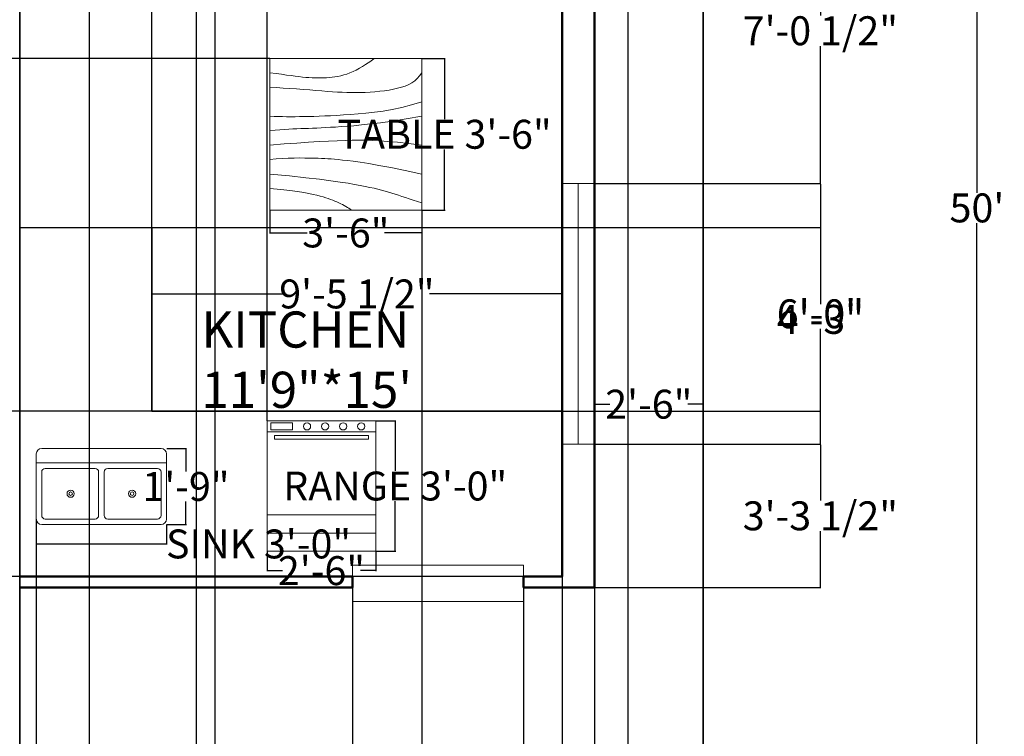
# Model space of a CAD drawing. Units: inches. Extents: x 3437 to 3994, y 3379 to 4084.
# Tile 4 of 6: x 3722 to 3994, y 3577 to 3776. Entities that reach past the tile are written whole.
import ezdxf

# ---------------------------------------------------------------- set-up
doc = ezdxf.new("R2010")
doc.units = ezdxf.units.IN
doc.header["$MEASUREMENT"] = 0
for name, color, linetype, lineweight in [('A-ANNO-DIMS', 2, 'Continuous', 18), ('A-AREA-IDEN', 7, 'Continuous', 25), ('A-EQPM', 8, 'Continuous', 18), ('A-FLOR-CASE', 8, 'Continuous', 25), ('A-FLOR-FIXT', 9, 'Continuous', 18), ('A-FURN', 8, 'Continuous', 18), ('A-GLAZ', 4, 'Continuous', 18), ('A-WALL', 7, 'Continuous', 50), ('C-PROP', 3, 'Continuous', 25)]:
    doc.layers.add(name, color=color, linetype=linetype, lineweight=lineweight)
doc.styles.get("Standard").update_dxf_attribs({"font": 'arial.ttf'})
doc.dimstyles.get("Standard").update_dxf_attribs({"dimtxt": 8, "dimasz": 0.18, "dimexe": 0.18, "dimexo": 0.0625, "dimgap": 0.09, "dimtad": 0, "dimtih": 1, "dimtoh": 1, "dimdec": 0, "dimzin": 0, "dimdsep": 46, "dimlunit": 3, "dimtxsty": 'Standard', "dimcen": 0.09, "dimadec": 0, "dimazin": 0, "dimtfac": 1, "dimtdec": 0, "dimtofl": 0, "dimtmove": 0, "dimatfit": 3, "dimfxl": 1, "dimtolj": 1, "dimtzin": 0, "dimarcsym": 0})

# ---------------------------------------------------------------- blocks, each defined once
blk = doc.blocks.new('Sink-double - 36 in top')
for p, q in [((-18, -4), (18, -4)), ((-0.75, -18.5), (-0.75, -6.5)), ((0.75, -6.5), (0.75, -18.5))]:
    blk.add_line(p, q)
for points in [[(-16.5, 0), (16.5, 0)], [(-18, -19.5), (-18, -1.5)], [(18, -1.5), (18, -19.5)], [(-16.5, -18.5), (-16.5, -6.5)], [(-15.5, -5.5), (-1.75, -5.5)], [(1.75, -5.5), (15.5, -5.5)], [(16.5, -6.5), (16.5, -18.5)], [(16.5, -21), (-16.5, -21)], [(-1.75, -19.5), (-15.5, -19.5)], [(15.5, -19.5), (1.75, -19.5)]]:
    blk.add_lwpolyline(points)
for centre, radius in [((-8.5, -12.5), 1), ((-8.5, -12.5), 0.5), ((8.5, -12.5), 1), ((8.5, -12.5), 0.5)]:
    blk.add_circle(centre, radius)
for centre, radius, start, end in [((-16.5, -1.5), 1.5, 90, 180), ((16.5, -1.5), 1.5, 0, 90), ((-15.5, -6.5), 1, 90, 180), ((-1.75, -6.5), 1, 0, 90), ((1.75, -6.5), 1, 90, 180), ((15.5, -6.5), 1, 0, 90), ((-15.5, -18.5), 1, 180, 270), ((-1.75, -18.5), 1, 270, 0), ((1.75, -18.5), 1, 180, 270), ((15.5, -18.5), 1, 270, 0), ((-16.5, -19.5), 1.5, 180, 270), ((16.5, -19.5), 1.5, 270, 0)]:
    blk.add_arc(centre, radius, start, end)
blk = doc.blocks.new('Range-Oven - 30 in front')
for p, q in [((0, 33.00005), (30, 33.00005)), ((30, 10), (0, 10)), ((0, 5), (30, 5))]:
    blk.add_line(p, q)
for points in [[(0, 0), (0, 36.00005), (30, 36.00005), (30, 0)], [(1, 33.50005), (1, 35.50005), (7, 35.50005), (7, 33.50005)], [(2, 31.00005), (2, 32.00005), (28, 32.00005), (28, 31.00005)]]:
    blk.add_lwpolyline(points, close=True)
for centre in [(11, 34.50005), (16, 34.50005), (21, 34.50005), (26, 34.50005)]:
    blk.add_circle(centre, 1)
blk = doc.blocks.new('Table - Square Woodgrain 42 x 42 in.')
blk.add_line((0, -42), (42, -42))
for points in [[(0, -4), (1.704, -4.2172), (3.2358, -4.4188), (4.615, -4.604), (5.8615, -4.7721), (6.9951, -4.9224), (8.0357, -5.0541), (9.0031, -5.1667), (9.9171, -5.2594), (10.7951, -5.3316), (11.6445, -5.3836), (12.4702, -5.4157), (13.277, -5.4283), (14.0698, -5.4217), (14.8535, -5.3964), (15.6331, -5.3526), (16.4133, -5.2908), (17.1986, -5.2103), (17.9913, -5.1062), (18.793, -4.9727), (19.6056, -4.8038), (20.4307, -4.5937), (21.2701, -4.3365), (22.1256, -4.0262), (22.9989, -3.6571), (23.888, -3.2272), (24.7756, -2.7516), (25.6408, -2.2491), (26.4624, -1.7387), (27.2195, -1.2395), (27.891, -0.7703), (28.456, -0.3501), (28.8934, 0.002)], [(0, -42), (0, 0), (42, 0), (42, -42)], [(0, -8), (1.8203, -8.1001), (3.6741, -8.2149), (5.5411, -8.3408), (7.4011, -8.4741), (9.2339, -8.6112), (11.0193, -8.7484), (12.7371, -8.8821), (14.3671, -9.0086), (15.8954, -9.1246), (17.3337, -9.2278), (18.6997, -9.3159), (20.0116, -9.387), (21.2871, -9.4389), (22.5442, -9.4696), (23.8008, -9.477), (25.0749, -9.459), (26.3791, -9.4137), (27.7049, -9.3403), (29.0383, -9.2382), (30.3655, -9.1068), (31.6728, -8.9455), (32.9461, -8.7535), (34.1717, -8.5304), (35.3358, -8.2756), (36.4268, -7.9863), (37.443, -7.6521), (38.3849, -7.2603), (39.253, -6.7986), (40.048, -6.2542), (40.7705, -5.6147), (41.421, -4.8674), (42, -4)], [(42, -12), (39.1784, -12.8621), (36.4519, -13.5654), (33.8246, -14.1294), (31.3004, -14.5731), (28.8832, -14.9161), (26.577, -15.1775), (24.3858, -15.3768), (22.3136, -15.5332), (20.3622, -15.6632), (18.5254, -15.7718), (16.7947, -15.8612), (15.1618, -15.9338), (13.6183, -15.9916), (12.1558, -16.0369), (10.7659, -16.0718), (9.4403, -16.0987), (8.1703, -16.1191), (6.9461, -16.1325), (5.7577, -16.1377), (4.595, -16.1335), (3.4479, -16.1188), (2.3064, -16.0924), (1.1604, -16.0532), (0, -16)], [(42, -16), (37.6529, -16.7365), (33.8802, -17.329), (30.6179, -17.7961), (27.8015, -18.1561), (25.3668, -18.4275), (23.2497, -18.6288), (21.3859, -18.7785), (19.7111, -18.8949), (18.1693, -18.9939), (16.7375, -19.0795), (15.401, -19.1534), (14.1449, -19.217), (12.9544, -19.2717), (11.8148, -19.3191), (10.7113, -19.3606), (9.6291, -19.3976), (8.5534, -19.4323), (7.47, -19.4689), (6.3643, -19.5122), (5.222, -19.5672), (4.0288, -19.6386), (2.7703, -19.7313), (1.4321, -19.8501), (0, -20)], [(0, -24), (3.9243, -23.6805), (7.4766, -23.4138), (10.6891, -23.1954), (13.5943, -23.0205), (16.2247, -22.8847), (18.6125, -22.7832), (20.7903, -22.7116), (22.7903, -22.6651), (24.6563, -22.642), (26.4764, -22.6507), (28.35, -22.7024), (30.3766, -22.8084), (32.6555, -22.98), (35.2861, -23.2283), (38.3678, -23.5645), (42, -24)], [(42, -32), (37.392, -31.017), (33.4585, -30.2231), (30.1291, -29.5949), (27.3334, -29.109), (25.0009, -28.742), (23.0612, -28.4707), (21.4439, -28.2716), (20.0786, -28.1215), (18.8998, -28.0002), (17.8609, -27.9014), (16.9206, -27.8219), (16.0371, -27.7588), (15.1691, -27.709), (14.2748, -27.6693), (13.3128, -27.6368), (12.2415, -27.6083), (11.0295, -27.5824), (9.6867, -27.5643), (8.233, -27.5608), (6.6884, -27.5787), (5.0728, -27.6248), (3.4062, -27.7058), (1.7086, -27.8286), (0, -28)], [(0, -32), (5.4026, -32.5358), (9.9494, -33.019), (13.7424, -33.4553), (16.8834, -33.8505), (19.4743, -34.2106), (21.6171, -34.5413), (23.4136, -34.8486), (24.9657, -35.1382), (26.3614, -35.4156), (27.6332, -35.6841), (28.7995, -35.9467), (29.8788, -36.2064), (30.8897, -36.4661), (31.8507, -36.7288), (32.7802, -36.9973), (33.6968, -37.2747), (34.6175, -37.5635), (35.5531, -37.8651), (36.5128, -38.1805), (37.506, -38.5108), (38.5421, -38.8568), (39.6302, -39.2197), (40.7797, -39.6004), (42, -40)], [(0, -36), (3.0098, -36.2857), (5.5354, -36.5643), (7.6368, -36.8359), (9.374, -37.1009), (10.807, -37.3597), (11.9957, -37.6126), (13.0002, -37.8599), (13.8804, -38.102), (14.6874, -38.3393), (15.4365, -38.5729), (16.1338, -38.8041), (16.7858, -39.0341), (17.3987, -39.264), (17.9787, -39.4952), (18.5322, -39.7288), (19.0655, -39.9662), (19.5832, -40.2081), (20.0842, -40.4544), (20.5657, -40.7046), (21.0249, -40.9581), (21.459, -41.2144), (21.8653, -41.4731), (22.2409, -41.7335), (22.5831, -41.9951)]]:
    blk.add_lwpolyline(points)
blk = doc.blocks.new('*D10')
at = {"layer": 'A-ANNO-DIMS', "color": 0, "lineweight": -2, "transparency": 16777216}
for p, q in [((3911.09, 4023.64), (3986.96, 4023.64)), ((3986.78, 4023.46), (3986.78, 3727.81)), ((3986.78, 3423.82), (3986.78, 3719.46)), ((3911.09, 3423.64), (3986.96, 3423.64))]:
    blk.add_line(p, q, dxfattribs=at)
at = {"layer": 'A-ANNO-DIMS', "color": 0, "transparency": 16777216}
for points in [[(3986.75, 4023.46), (3986.81, 4023.46), (3986.78, 4023.64)], [(3986.75, 3423.82), (3986.81, 3423.82), (3986.78, 3423.64)]]:
    blk.add_solid(points, dxfattribs=at)
at = {"layer": 'Defpoints', "color": 0, "transparency": 16777216}
for p in [(3911.02, 4023.64), (3986.78, 4023.64), (3911.02, 3423.64)]:
    blk.add_point(p, dxfattribs=at)
at = {"layer": 'A-ANNO-DIMS', "color": 0, "transparency": 16777216, "insert": (3986.78, 3723.64), "char_height": 8, "attachment_point": 5}
blk.add_mtext("\\A1;50'", dxfattribs=at)
blk = doc.blocks.new('*D11')
at = {"layer": 'A-ANNO-DIMS', "color": 0, "lineweight": -2, "transparency": 16777216}
for p, q in [((3881.02, 3665.86), (3881.02, 3669.53)), ((3881.2, 3669.35), (3885.23, 3669.35)), ((3910.84, 3669.35), (3906.82, 3669.35)), ((3911.02, 3665.86), (3911.02, 3669.53))]:
    blk.add_line(p, q, dxfattribs=at)
at = {"layer": 'A-ANNO-DIMS', "color": 0, "transparency": 16777216}
for points in [[(3881.2, 3669.38), (3881.2, 3669.32), (3881.02, 3669.35)], [(3910.84, 3669.38), (3910.84, 3669.32), (3911.02, 3669.35)]]:
    blk.add_solid(points, dxfattribs=at)
at = {"layer": 'Defpoints', "color": 0, "transparency": 16777216}
for p in [(3911.02, 3669.35), (3881.02, 3665.8), (3911.02, 3665.8)]:
    blk.add_point(p, dxfattribs=at)
at = {"layer": 'A-ANNO-DIMS', "color": 0, "transparency": 16777216, "insert": (3896.02, 3669.35), "char_height": 8, "attachment_point": 5}
blk.add_mtext('\\A1;2\'-6"', dxfattribs=at)
blk = doc.blocks.new('*D17')
at = {"layer": 'A-ANNO-DIMS', "color": 0, "lineweight": -2, "transparency": 16777216}
for p, q in [((3726.61, 3636.03), (3726.61, 3630.51)), ((3762.61, 3636.03), (3762.61, 3630.51)), ((3726.79, 3630.69), (3762.43, 3630.69)), ((3762.61, 3630.69), (3762.79, 3630.69))]:
    blk.add_line(p, q, dxfattribs=at)
at = {"layer": 'A-ANNO-DIMS', "color": 0, "transparency": 16777216}
for points in [[(3726.79, 3630.72), (3726.79, 3630.66), (3726.61, 3630.69)], [(3762.43, 3630.72), (3762.43, 3630.66), (3762.61, 3630.69)]]:
    blk.add_solid(points, dxfattribs=at)
at = {"layer": 'Defpoints', "color": 0, "transparency": 16777216}
for p in [(3726.61, 3636.09), (3762.61, 3636.09), (3762.61, 3630.69)]:
    blk.add_point(p, dxfattribs=at)
at = {"layer": 'A-ANNO-DIMS', "color": 0, "transparency": 16777216, "insert": (3788.09, 3630.69), "char_height": 8, "attachment_point": 5}
blk.add_mtext('\\A1;SINK 3\'-0"', dxfattribs=at)
blk = doc.blocks.new('*D18')
at = {"layer": 'A-ANNO-DIMS', "color": 0, "lineweight": -2, "transparency": 16777216}
for p, q in [((3762.68, 3657.09), (3768.19, 3657.09)), ((3768.01, 3656.91), (3768.01, 3650.77)), ((3768.01, 3636.27), (3768.01, 3642.42)), ((3762.68, 3636.09), (3768.19, 3636.09))]:
    blk.add_line(p, q, dxfattribs=at)
at = {"layer": 'A-ANNO-DIMS', "color": 0, "transparency": 16777216}
for points in [[(3767.98, 3656.91), (3768.04, 3656.91), (3768.01, 3657.09)], [(3767.98, 3636.27), (3768.04, 3636.27), (3768.01, 3636.09)]]:
    blk.add_solid(points, dxfattribs=at)
at = {"layer": 'Defpoints', "color": 0, "transparency": 16777216}
for p in [(3762.61, 3657.09), (3768.01, 3657.09), (3762.61, 3636.09)]:
    blk.add_point(p, dxfattribs=at)
at = {"layer": 'A-ANNO-DIMS', "color": 0, "transparency": 16777216, "insert": (3768.01, 3646.59), "char_height": 8, "attachment_point": 5}
blk.add_mtext('\\A1;1\'-9"', dxfattribs=at)
blk = doc.blocks.new('*D19')
at = {"layer": 'A-ANNO-DIMS', "color": 0, "lineweight": -2, "transparency": 16777216}
for p, q in [((3820.55, 3664.71), (3826.07, 3664.71)), ((3825.89, 3664.53), (3825.89, 3650.94)), ((3825.89, 3628.89), (3825.89, 3642.48)), ((3820.55, 3628.71), (3826.07, 3628.71))]:
    blk.add_line(p, q, dxfattribs=at)
at = {"layer": 'A-ANNO-DIMS', "color": 0, "transparency": 16777216}
for points in [[(3825.86, 3664.53), (3825.92, 3664.53), (3825.89, 3664.71)], [(3825.86, 3628.89), (3825.92, 3628.89), (3825.89, 3628.71)]]:
    blk.add_solid(points, dxfattribs=at)
at = {"layer": 'Defpoints', "color": 0, "transparency": 16777216}
for p in [(3820.49, 3664.71), (3825.89, 3664.71), (3820.49, 3628.71)]:
    blk.add_point(p, dxfattribs=at)
at = {"layer": 'A-ANNO-DIMS', "color": 0, "transparency": 16777216, "insert": (3825.89, 3646.71), "char_height": 8, "attachment_point": 5}
blk.add_mtext('\\A1;RANGE 3\'-0"', dxfattribs=at)
blk = doc.blocks.new('*D20')
at = {"layer": 'A-ANNO-DIMS', "color": 0, "lineweight": -2, "transparency": 16777216}
for p, q in [((3790.49, 3628.64), (3790.49, 3623.13)), ((3820.49, 3628.64), (3820.49, 3623.13)), ((3790.67, 3623.31), (3794.69, 3623.31)), ((3820.31, 3623.31), (3816.28, 3623.31))]:
    blk.add_line(p, q, dxfattribs=at)
at = {"layer": 'A-ANNO-DIMS', "color": 0, "transparency": 16777216}
for points in [[(3790.67, 3623.34), (3790.67, 3623.28), (3790.49, 3623.31)], [(3820.31, 3623.34), (3820.31, 3623.28), (3820.49, 3623.31)]]:
    blk.add_solid(points, dxfattribs=at)
at = {"layer": 'Defpoints', "color": 0, "transparency": 16777216}
for p in [(3790.49, 3628.71), (3820.49, 3628.71), (3820.49, 3623.31)]:
    blk.add_point(p, dxfattribs=at)
at = {"layer": 'A-ANNO-DIMS', "color": 0, "transparency": 16777216, "insert": (3805.49, 3623.31), "char_height": 8, "attachment_point": 5}
blk.add_mtext('\\A1;2\'-6"', dxfattribs=at)
blk = doc.blocks.new('*D23')
at = {"layer": 'A-ANNO-DIMS', "color": 0, "lineweight": -2, "transparency": 16777216}
for p, q in [((3833.29, 3765.01), (3839.71, 3765.01)), ((3839.53, 3764.83), (3839.53, 3748.19)), ((3839.53, 3723.19), (3839.53, 3739.83)), ((3833.29, 3723.01), (3839.71, 3723.01))]:
    blk.add_line(p, q, dxfattribs=at)
at = {"layer": 'A-ANNO-DIMS', "color": 0, "transparency": 16777216}
for points in [[(3839.5, 3764.83), (3839.56, 3764.83), (3839.53, 3765.01)], [(3839.5, 3723.19), (3839.56, 3723.19), (3839.53, 3723.01)]]:
    blk.add_solid(points, dxfattribs=at)
at = {"layer": 'Defpoints', "color": 0, "transparency": 16777216}
for p in [(3833.23, 3765.01), (3839.53, 3765.01), (3833.23, 3723.01)]:
    blk.add_point(p, dxfattribs=at)
at = {"layer": 'A-ANNO-DIMS', "color": 0, "transparency": 16777216, "insert": (3839.53, 3744.01), "char_height": 8, "attachment_point": 5}
blk.add_mtext('\\A1;TABLE 3\'-6"', dxfattribs=at)
blk = doc.blocks.new('*D24')
at = {"layer": 'A-ANNO-DIMS', "color": 0, "lineweight": -2, "transparency": 16777216}
for p, q in [((3791.23, 3722.95), (3791.23, 3716.53)), ((3833.23, 3722.95), (3833.23, 3716.53)), ((3791.41, 3716.71), (3801.51, 3716.71)), ((3833.05, 3716.71), (3822.95, 3716.71))]:
    blk.add_line(p, q, dxfattribs=at)
at = {"layer": 'A-ANNO-DIMS', "color": 0, "transparency": 16777216}
for points in [[(3791.41, 3716.74), (3791.41, 3716.68), (3791.23, 3716.71)], [(3833.05, 3716.74), (3833.05, 3716.68), (3833.23, 3716.71)]]:
    blk.add_solid(points, dxfattribs=at)
at = {"layer": 'Defpoints', "color": 0, "transparency": 16777216}
for p in [(3791.23, 3723.01), (3833.23, 3723.01), (3833.23, 3716.71)]:
    blk.add_point(p, dxfattribs=at)
at = {"layer": 'A-ANNO-DIMS', "color": 0, "transparency": 16777216, "insert": (3812.23, 3716.71), "char_height": 8, "attachment_point": 5}
blk.add_mtext('\\A1;3\'-6"', dxfattribs=at)
blk = doc.blocks.new('*D43')
at = {"layer": 'A-ANNO-DIMS', "color": 0, "lineweight": -2, "transparency": 16777216}
for p, q in [((3881.09, 3814.92), (3943.65, 3814.92)), ((3943.47, 3814.74), (3943.47, 3776.88)), ((3943.47, 3730.56), (3943.47, 3768.42)), ((3881.09, 3730.38), (3943.65, 3730.38))]:
    blk.add_line(p, q, dxfattribs=at)
at = {"layer": 'A-ANNO-DIMS', "color": 0, "transparency": 16777216}
for points in [[(3943.44, 3814.74), (3943.5, 3814.74), (3943.47, 3814.92)], [(3943.44, 3730.56), (3943.5, 3730.56), (3943.47, 3730.38)]]:
    blk.add_solid(points, dxfattribs=at)
at = {"layer": 'Defpoints', "color": 0, "transparency": 16777216}
for p in [(3881.02, 3814.92), (3881.02, 3730.38), (3943.47, 3730.38)]:
    blk.add_point(p, dxfattribs=at)
at = {"layer": 'A-ANNO-DIMS', "color": 0, "transparency": 16777216, "insert": (3943.47, 3772.65), "char_height": 8, "attachment_point": 5}
blk.add_mtext('\\A1;7\'-0 1/2"', dxfattribs=at)
blk = doc.blocks.new('*D44')
at = {"layer": 'A-ANNO-DIMS', "color": 0, "lineweight": -2, "transparency": 16777216}
for p, q in [((3881.09, 3730.38), (3943.65, 3730.38)), ((3943.47, 3730.2), (3943.47, 3698.52)), ((3943.47, 3658.49), (3943.47, 3690.17)), ((3881.09, 3658.31), (3943.65, 3658.31))]:
    blk.add_line(p, q, dxfattribs=at)
at = {"layer": 'A-ANNO-DIMS', "color": 0, "transparency": 16777216}
for points in [[(3943.44, 3730.2), (3943.5, 3730.2), (3943.47, 3730.38)], [(3943.44, 3658.49), (3943.5, 3658.49), (3943.47, 3658.31)]]:
    blk.add_solid(points, dxfattribs=at)
at = {"layer": 'Defpoints', "color": 0, "transparency": 16777216}
for p in [(3881.02, 3730.38), (3881.02, 3658.31), (3943.47, 3658.31)]:
    blk.add_point(p, dxfattribs=at)
at = {"layer": 'A-ANNO-DIMS', "color": 0, "transparency": 16777216, "insert": (3943.47, 3694.35), "char_height": 8, "attachment_point": 5}
blk.add_mtext('\\A1;6\'-0"', dxfattribs=at)
blk = doc.blocks.new('*D45')
at = {"layer": 'A-ANNO-DIMS', "color": 0, "lineweight": -2, "transparency": 16777216}
for p, q in [((3881.09, 3658.31), (3943.65, 3658.31)), ((3943.47, 3658.13), (3943.47, 3642.7)), ((3943.47, 3618.82), (3943.47, 3634.25)), ((3881.09, 3618.64), (3943.65, 3618.64))]:
    blk.add_line(p, q, dxfattribs=at)
at = {"layer": 'A-ANNO-DIMS', "color": 0, "transparency": 16777216}
for points in [[(3943.44, 3658.13), (3943.5, 3658.13), (3943.47, 3658.31)], [(3943.44, 3618.82), (3943.5, 3618.82), (3943.47, 3618.64)]]:
    blk.add_solid(points, dxfattribs=at)
at = {"layer": 'Defpoints', "color": 0, "transparency": 16777216}
for p in [(3881.02, 3658.31), (3881.02, 3618.64), (3943.47, 3618.64)]:
    blk.add_point(p, dxfattribs=at)
at = {"layer": 'A-ANNO-DIMS', "color": 0, "transparency": 16777216, "insert": (3943.47, 3638.47), "char_height": 8, "attachment_point": 5}
blk.add_mtext('\\A1;3\'-3 1/2"', dxfattribs=at)
blk = doc.blocks.new('*D46')
at = {"layer": 'A-ANNO-DIMS', "color": 0, "lineweight": -2, "transparency": 16777216}
for p, q in [((3576.02, 3426.7), (3576.02, 4056.27)), ((3576.2, 4056.09), (3635.57, 4056.09)), ((3721.84, 4056.09), (3662.48, 4056.09)), ((3722.02, 3426.7), (3722.02, 4056.27))]:
    blk.add_line(p, q, dxfattribs=at)
at = {"layer": 'A-ANNO-DIMS', "color": 0, "transparency": 16777216}
for points in [[(3576.2, 4056.12), (3576.2, 4056.06), (3576.02, 4056.09)], [(3721.84, 4056.12), (3721.84, 4056.06), (3722.02, 4056.09)]]:
    blk.add_solid(points, dxfattribs=at)
at = {"layer": 'Defpoints', "color": 0, "transparency": 16777216}
for p in [(3722.02, 4056.09), (3576.02, 3426.64), (3722.02, 3426.64)]:
    blk.add_point(p, dxfattribs=at)
at = {"layer": 'A-ANNO-DIMS', "color": 0, "transparency": 16777216, "insert": (3649.02, 4056.09), "char_height": 8, "attachment_point": 5}
blk.add_mtext('\\A1;12\'-2"', dxfattribs=at)
blk = doc.blocks.new('*D48')
at = {"layer": 'A-ANNO-DIMS', "color": 0, "lineweight": -2, "transparency": 16777216}
for p, q in [((3722.02, 3861.57), (3722.02, 3391.01)), ((3719.02, 3858.57), (3719.02, 3391.01)), ((3719.2, 3391.19), (3721.84, 3391.19)), ((3722.02, 3391.19), (3722.2, 3391.19))]:
    blk.add_line(p, q, dxfattribs=at)
at = {"layer": 'A-ANNO-DIMS', "color": 0, "transparency": 16777216}
for points in [[(3719.2, 3391.22), (3719.2, 3391.16), (3719.02, 3391.19)], [(3721.84, 3391.22), (3721.84, 3391.16), (3722.02, 3391.19)]]:
    blk.add_solid(points, dxfattribs=at)
at = {"layer": 'Defpoints', "color": 0, "transparency": 16777216}
for p in [(3722.02, 3861.64), (3719.02, 3858.64), (3722.02, 3391.19)]:
    blk.add_point(p, dxfattribs=at)
at = {"layer": 'A-ANNO-DIMS', "color": 0, "transparency": 16777216, "insert": (3732.93, 3391.19), "char_height": 8, "attachment_point": 5}
blk.add_mtext('\\A1;0\'-3"', dxfattribs=at)
blk = doc.blocks.new('*D51')
at = {"layer": 'A-ANNO-DIMS', "color": 0, "lineweight": -2, "transparency": 16777216}
for p, q in [((3814.05, 3618.57), (3814.05, 3391.01)), ((3861.41, 3618.57), (3861.41, 3391.01)), ((3814.23, 3391.19), (3814.58, 3391.19)), ((3861.23, 3391.19), (3860.88, 3391.19))]:
    blk.add_line(p, q, dxfattribs=at)
at = {"layer": 'A-ANNO-DIMS', "color": 0, "transparency": 16777216}
for points in [[(3814.23, 3391.22), (3814.23, 3391.16), (3814.05, 3391.19)], [(3861.23, 3391.22), (3861.23, 3391.16), (3861.41, 3391.19)]]:
    blk.add_solid(points, dxfattribs=at)
at = {"layer": 'Defpoints', "color": 0, "transparency": 16777216}
for p in [(3814.05, 3618.64), (3861.41, 3618.64), (3861.41, 3391.19)]:
    blk.add_point(p, dxfattribs=at)
at = {"layer": 'A-ANNO-DIMS', "color": 0, "transparency": 16777216, "insert": (3837.73, 3391.19), "char_height": 8, "attachment_point": 5}
blk.add_mtext('\\A1;3\'-11 1/2"', dxfattribs=at)
blk = doc.blocks.new('*D52')
at = {"layer": 'A-ANNO-DIMS', "color": 0, "lineweight": -2, "transparency": 16777216}
for p, q in [((3861.41, 3618.57), (3861.41, 3391.01)), ((3881.02, 3618.57), (3881.02, 3391.01)), ((3861.59, 3391.19), (3880.84, 3391.19)), ((3881.02, 3391.19), (3881.2, 3391.19))]:
    blk.add_line(p, q, dxfattribs=at)
at = {"layer": 'A-ANNO-DIMS', "color": 0, "transparency": 16777216}
for points in [[(3861.59, 3391.22), (3861.59, 3391.16), (3861.41, 3391.19)], [(3880.84, 3391.22), (3880.84, 3391.16), (3881.02, 3391.19)]]:
    blk.add_solid(points, dxfattribs=at)
at = {"layer": 'Defpoints', "color": 0, "transparency": 16777216}
for p in [(3861.41, 3618.64), (3881.02, 3618.64), (3881.02, 3391.19)]:
    blk.add_point(p, dxfattribs=at)
at = {"layer": 'A-ANNO-DIMS', "color": 0, "transparency": 16777216, "insert": (3900.87, 3391.19), "char_height": 8, "attachment_point": 5}
blk.add_mtext('\\A1;1\'-7 1/2"', dxfattribs=at)
blk = doc.blocks.new('*D53')
at = {"layer": 'A-ANNO-DIMS', "color": 0, "lineweight": -2, "transparency": 16777216}
for p, q in [((3770.9, 3426.7), (3770.9, 4056.27)), ((3771.08, 4056.09), (3807.48, 4056.09)), ((3890.18, 4056.09), (3853.78, 4056.09)), ((3890.36, 3426.7), (3890.36, 4056.27))]:
    blk.add_line(p, q, dxfattribs=at)
at = {"layer": 'A-ANNO-DIMS', "color": 0, "transparency": 16777216}
for points in [[(3771.08, 4056.12), (3771.08, 4056.06), (3770.9, 4056.09)], [(3890.18, 4056.12), (3890.18, 4056.06), (3890.36, 4056.09)]]:
    blk.add_solid(points, dxfattribs=at)
at = {"layer": 'Defpoints', "color": 0, "transparency": 16777216}
for p in [(3890.36, 4056.09), (3770.9, 3426.64), (3890.36, 3426.64)]:
    blk.add_point(p, dxfattribs=at)
at = {"layer": 'A-ANNO-DIMS', "color": 0, "transparency": 16777216, "insert": (3830.63, 4056.09), "char_height": 8, "attachment_point": 5}
blk.add_mtext('\\A1;9\'-11 1/2"', dxfattribs=at)
blk = doc.blocks.new('*D54')
at = {"layer": 'A-ANNO-DIMS', "color": 0, "lineweight": -2, "transparency": 16777216}
for p, q in [((3890.36, 3426.7), (3890.36, 4056.27)), ((3890.54, 4056.09), (3910.84, 4056.09)), ((3911.02, 3426.7), (3911.02, 4056.27)), ((3911.02, 4056.09), (3911.2, 4056.09))]:
    blk.add_line(p, q, dxfattribs=at)
at = {"layer": 'A-ANNO-DIMS', "color": 0, "transparency": 16777216}
for points in [[(3890.54, 4056.12), (3890.54, 4056.06), (3890.36, 4056.09)], [(3910.84, 4056.12), (3910.84, 4056.06), (3911.02, 4056.09)]]:
    blk.add_solid(points, dxfattribs=at)
at = {"layer": 'Defpoints', "color": 0, "transparency": 16777216}
for p in [(3911.02, 4056.09), (3890.36, 3426.64), (3911.02, 3426.64)]:
    blk.add_point(p, dxfattribs=at)
at = {"layer": 'A-ANNO-DIMS', "color": 0, "transparency": 16777216, "insert": (3930.87, 4056.09), "char_height": 8, "attachment_point": 5}
blk.add_mtext('\\A1;1\'-8 1/2"', dxfattribs=at)
blk = doc.blocks.new('*D57')
at = {"layer": 'A-ANNO-DIMS', "color": 0, "lineweight": -2, "transparency": 16777216}
for p, q in [((3741.22, 3861.57), (3741.22, 3391.01)), ((3776.02, 3861.57), (3776.02, 3391.01)), ((3741.4, 3391.19), (3744.72, 3391.19)), ((3775.84, 3391.19), (3772.52, 3391.19))]:
    blk.add_line(p, q, dxfattribs=at)
at = {"layer": 'A-ANNO-DIMS', "color": 0, "transparency": 16777216}
for points in [[(3741.4, 3391.22), (3741.4, 3391.16), (3741.22, 3391.19)], [(3775.84, 3391.22), (3775.84, 3391.16), (3776.02, 3391.19)]]:
    blk.add_solid(points, dxfattribs=at)
at = {"layer": 'Defpoints', "color": 0, "transparency": 16777216}
for p in [(3741.22, 3861.64), (3776.02, 3861.64), (3776.02, 3391.19)]:
    blk.add_point(p, dxfattribs=at)
at = {"layer": 'A-ANNO-DIMS', "color": 0, "transparency": 16777216, "insert": (3758.62, 3391.19), "char_height": 8, "attachment_point": 5}
blk.add_mtext('\\A1;2\'-11"', dxfattribs=at)
blk = doc.blocks.new('*D64')
at = {"layer": 'A-ANNO-DIMS', "color": 0, "lineweight": -2, "transparency": 16777216}
for p, q in [((3722.02, 3718.27), (3722.02, 4056.27)), ((3722.2, 4056.09), (3758.36, 4056.09)), ((3758.54, 3718.27), (3758.54, 4056.27)), ((3758.54, 4056.09), (3758.72, 4056.09))]:
    blk.add_line(p, q, dxfattribs=at)
at = {"layer": 'A-ANNO-DIMS', "color": 0, "transparency": 16777216}
for points in [[(3722.2, 4056.12), (3722.2, 4056.06), (3722.02, 4056.09)], [(3758.36, 4056.12), (3758.36, 4056.06), (3758.54, 4056.09)]]:
    blk.add_solid(points, dxfattribs=at)
at = {"layer": 'Defpoints', "color": 0, "transparency": 16777216}
for p in [(3758.54, 4056.09), (3722.02, 3718.21), (3758.54, 3718.21)]:
    blk.add_point(p, dxfattribs=at)
at = {"layer": 'A-ANNO-DIMS', "color": 0, "transparency": 16777216, "insert": (3778.76, 4056.09), "char_height": 8, "attachment_point": 5}
blk.add_mtext('\\A1;3\'-0 1/2"', dxfattribs=at)
blk = doc.blocks.new('*D65')
at = {"layer": 'A-ANNO-DIMS', "color": 0, "lineweight": -2, "transparency": 16777216}
for p, q in [((3758.6, 3718.21), (3943.65, 3718.21)), ((3943.47, 3718.03), (3943.47, 3696.98)), ((3943.47, 3667.57), (3943.47, 3688.62)), ((3758.6, 3667.39), (3943.65, 3667.39))]:
    blk.add_line(p, q, dxfattribs=at)
at = {"layer": 'A-ANNO-DIMS', "color": 0, "transparency": 16777216}
for points in [[(3943.44, 3718.03), (3943.5, 3718.03), (3943.47, 3718.21)], [(3943.44, 3667.57), (3943.5, 3667.57), (3943.47, 3667.39)]]:
    blk.add_solid(points, dxfattribs=at)
at = {"layer": 'Defpoints', "color": 0, "transparency": 16777216}
for p in [(3758.54, 3718.21), (3943.47, 3718.21), (3758.54, 3667.39)]:
    blk.add_point(p, dxfattribs=at)
at = {"layer": 'A-ANNO-DIMS', "color": 0, "transparency": 16777216, "insert": (3943.47, 3692.8), "char_height": 8, "attachment_point": 5}
blk.add_mtext('\\A1;4\'-3"', dxfattribs=at)
blk = doc.blocks.new('*D66')
at = {"layer": 'A-ANNO-DIMS', "color": 0, "lineweight": -2, "transparency": 16777216}
for p, q in [((3871.96, 3667.39), (3458.39, 3667.39)), ((3458.57, 3667.21), (3458.57, 3648.69)), ((3458.57, 3621.82), (3458.57, 3640.34)), ((3871.96, 3621.64), (3458.39, 3621.64))]:
    blk.add_line(p, q, dxfattribs=at)
at = {"layer": 'A-ANNO-DIMS', "color": 0, "transparency": 16777216}
for points in [[(3458.54, 3667.21), (3458.6, 3667.21), (3458.57, 3667.39)], [(3458.54, 3621.82), (3458.6, 3621.82), (3458.57, 3621.64)]]:
    blk.add_solid(points, dxfattribs=at)
at = {"layer": 'Defpoints', "color": 0, "transparency": 16777216}
for p in [(3458.57, 3667.39), (3872.02, 3667.39), (3872.02, 3621.64)]:
    blk.add_point(p, dxfattribs=at)
at = {"layer": 'A-ANNO-DIMS', "color": 0, "transparency": 16777216, "insert": (3458.57, 3644.51), "char_height": 8, "attachment_point": 5}
blk.add_mtext('\\A1;3\'-10"', dxfattribs=at)
blk = doc.blocks.new('*D79')
at = {"layer": 'A-ANNO-DIMS', "color": 0, "lineweight": -2, "transparency": 16777216}
for p, q in [((3675.76, 3905.25), (3675.76, 3391.01)), ((3665.02, 3903.57), (3665.02, 3391.01)), ((3665.2, 3391.19), (3675.58, 3391.19)), ((3675.76, 3391.19), (3675.94, 3391.19))]:
    blk.add_line(p, q, dxfattribs=at)
at = {"layer": 'A-ANNO-DIMS', "color": 0, "transparency": 16777216}
for points in [[(3665.2, 3391.22), (3665.2, 3391.16), (3665.02, 3391.19)], [(3675.58, 3391.22), (3675.58, 3391.16), (3675.76, 3391.19)]]:
    blk.add_solid(points, dxfattribs=at)
at = {"layer": 'Defpoints', "color": 0, "transparency": 16777216}
for p in [(3675.76, 3905.31), (3665.02, 3903.64), (3675.76, 3391.19)]:
    blk.add_point(p, dxfattribs=at)
at = {"layer": 'A-ANNO-DIMS', "color": 0, "transparency": 16777216, "insert": (3699.09, 3391.19), "char_height": 8, "attachment_point": 5}
blk.add_mtext('\\A1;0\'-10 1/2"', dxfattribs=at)
blk = doc.blocks.new('*D81')
at = {"layer": 'A-ANNO-DIMS', "color": 0, "lineweight": -2, "transparency": 16777216}
for p, q in [((3722.02, 3984.57), (3722.02, 3391.01)), ((3872.02, 3984.57), (3872.02, 3391.01)), ((3722.2, 3391.19), (3783.57, 3391.19)), ((3871.84, 3391.19), (3810.48, 3391.19))]:
    blk.add_line(p, q, dxfattribs=at)
at = {"layer": 'A-ANNO-DIMS', "color": 0, "transparency": 16777216}
for points in [[(3722.2, 3391.22), (3722.2, 3391.16), (3722.02, 3391.19)], [(3871.84, 3391.22), (3871.84, 3391.16), (3872.02, 3391.19)]]:
    blk.add_solid(points, dxfattribs=at)
at = {"layer": 'Defpoints', "color": 0, "transparency": 16777216}
for p in [(3722.02, 3984.64), (3872.02, 3984.64), (3872.02, 3391.19)]:
    blk.add_point(p, dxfattribs=at)
at = {"layer": 'A-ANNO-DIMS', "color": 0, "transparency": 16777216, "insert": (3797.02, 3391.19), "char_height": 8, "attachment_point": 5}
blk.add_mtext('\\A1;12\'-6"', dxfattribs=at)
blk = doc.blocks.new('*D82')
at = {"layer": 'A-ANNO-DIMS', "color": 0, "lineweight": -2, "transparency": 16777216}
for p, q in [((3758.54, 3667.46), (3758.54, 3700.02)), ((3758.72, 3699.84), (3795.24, 3699.84)), ((3871.84, 3699.84), (3835.33, 3699.84)), ((3872.02, 3667.46), (3872.02, 3700.02))]:
    blk.add_line(p, q, dxfattribs=at)
at = {"layer": 'A-ANNO-DIMS', "color": 0, "transparency": 16777216}
for points in [[(3758.72, 3699.87), (3758.72, 3699.81), (3758.54, 3699.84)], [(3871.84, 3699.87), (3871.84, 3699.81), (3872.02, 3699.84)]]:
    blk.add_solid(points, dxfattribs=at)
at = {"layer": 'Defpoints', "color": 0, "transparency": 16777216}
for p in [(3872.02, 3699.84), (3758.54, 3667.39), (3872.02, 3667.39)]:
    blk.add_point(p, dxfattribs=at)
at = {"layer": 'A-ANNO-DIMS', "color": 0, "transparency": 16777216, "insert": (3815.28, 3699.84), "char_height": 8, "attachment_point": 5}
blk.add_mtext('\\A1;9\'-5 1/2"', dxfattribs=at)
blk = doc.blocks.new('*D83')
at = {"layer": 'A-ANNO-DIMS', "color": 0, "lineweight": -2, "transparency": 16777216}
for p, q in [((3758.54, 3667.46), (3758.54, 4056.27)), ((3758.72, 4056.09), (3763.72, 4056.09)), ((3790.31, 4056.09), (3785.3, 4056.09)), ((3790.49, 3664.77), (3790.49, 4056.27))]:
    blk.add_line(p, q, dxfattribs=at)
at = {"layer": 'A-ANNO-DIMS', "color": 0, "transparency": 16777216}
for points in [[(3758.72, 4056.12), (3758.72, 4056.06), (3758.54, 4056.09)], [(3790.31, 4056.12), (3790.31, 4056.06), (3790.49, 4056.09)]]:
    blk.add_solid(points, dxfattribs=at)
at = {"layer": 'Defpoints', "color": 0, "transparency": 16777216}
for p in [(3790.49, 4056.09), (3758.54, 3667.39), (3790.49, 3664.71)]:
    blk.add_point(p, dxfattribs=at)
at = {"layer": 'A-ANNO-DIMS', "color": 0, "transparency": 16777216, "insert": (3774.51, 4056.09), "char_height": 8, "attachment_point": 5}
blk.add_mtext('\\A1;2\'-8"', dxfattribs=at)
blk = doc.blocks.new('*D84')
at = {"layer": 'A-ANNO-DIMS', "color": 0, "lineweight": -2, "transparency": 16777216}
for p, q in [((3726.61, 3637.53), (3726.61, 3391.01)), ((3722.02, 3621.57), (3722.02, 3391.01)), ((3722.2, 3391.19), (3726.43, 3391.19)), ((3726.61, 3391.19), (3726.79, 3391.19))]:
    blk.add_line(p, q, dxfattribs=at)
at = {"layer": 'A-ANNO-DIMS', "color": 0, "transparency": 16777216}
for points in [[(3722.2, 3391.22), (3722.2, 3391.16), (3722.02, 3391.19)], [(3726.43, 3391.22), (3726.43, 3391.16), (3726.61, 3391.19)]]:
    blk.add_solid(points, dxfattribs=at)
at = {"layer": 'Defpoints', "color": 0, "transparency": 16777216}
for p in [(3726.61, 3637.59), (3722.02, 3621.64), (3726.61, 3391.19)]:
    blk.add_point(p, dxfattribs=at)
at = {"layer": 'A-ANNO-DIMS', "color": 0, "transparency": 16777216, "insert": (3746.84, 3391.19), "char_height": 8, "attachment_point": 5}
blk.add_mtext('\\A1;0\'-4 1/2"', dxfattribs=at)
blk = doc.blocks.new('*D85')
at = {"layer": 'A-ANNO-DIMS', "color": 0, "lineweight": -2, "transparency": 16777216}
for p, q in [((3872.02, 3730.32), (3872.02, 3391.01)), ((3833.23, 3722.95), (3833.23, 3391.01)), ((3833.41, 3391.19), (3841.91, 3391.19)), ((3871.84, 3391.19), (3863.35, 3391.19))]:
    blk.add_line(p, q, dxfattribs=at)
at = {"layer": 'A-ANNO-DIMS', "color": 0, "transparency": 16777216}
for points in [[(3833.41, 3391.22), (3833.41, 3391.16), (3833.23, 3391.19)], [(3871.84, 3391.22), (3871.84, 3391.16), (3872.02, 3391.19)]]:
    blk.add_solid(points, dxfattribs=at)
at = {"layer": 'Defpoints', "color": 0, "transparency": 16777216}
for p in [(3872.02, 3730.38), (3833.23, 3723.01), (3872.02, 3391.19)]:
    blk.add_point(p, dxfattribs=at)
at = {"layer": 'A-ANNO-DIMS', "color": 0, "transparency": 16777216, "insert": (3852.63, 3391.19), "char_height": 8, "attachment_point": 5}
blk.add_mtext('\\A1;3\'-3"', dxfattribs=at)
blk = doc.blocks.new('*D86')
at = {"layer": 'A-ANNO-DIMS', "color": 0, "lineweight": -2, "transparency": 16777216}
for p, q in [((3775.96, 3798.64), (3458.39, 3798.64)), ((3458.57, 3798.46), (3458.57, 3786.05)), ((3458.57, 3765.19), (3458.57, 3777.6)), ((3791.17, 3765.01), (3458.39, 3765.01))]:
    blk.add_line(p, q, dxfattribs=at)
at = {"layer": 'A-ANNO-DIMS', "color": 0, "transparency": 16777216}
for points in [[(3458.54, 3798.46), (3458.6, 3798.46), (3458.57, 3798.64)], [(3458.54, 3765.19), (3458.6, 3765.19), (3458.57, 3765.01)]]:
    blk.add_solid(points, dxfattribs=at)
at = {"layer": 'Defpoints', "color": 0, "transparency": 16777216}
for p in [(3776.02, 3798.64), (3458.57, 3765.01), (3791.23, 3765.01)]:
    blk.add_point(p, dxfattribs=at)
at = {"layer": 'A-ANNO-DIMS', "color": 0, "transparency": 16777216, "insert": (3458.57, 3781.82), "char_height": 8, "attachment_point": 5}
blk.add_mtext('\\A1;2\'-9 1/2"', dxfattribs=at)

msp = doc.modelspace()

# ---------------------------------------------------------------- linework, layer by layer
at = {"layer": 'A-FLOR-CASE'}
for p, q in [((3722.02, 3718.21), (3758.54, 3718.21)), ((3758.54, 3718.21), (3758.54, 3667.39)), ((3758.54, 3667.39), (3872.02, 3667.39))]:
    msp.add_line(p, q, dxfattribs=at)
at = {"layer": 'A-GLAZ'}
for p, q in [((3872.02, 3730.38), (3881.02, 3730.38)), ((3876.52, 3730.38), (3876.52, 3658.31)), ((3872.02, 3658.31), (3881.02, 3658.31)), ((3814.05, 3621.64), (3814.05, 3624.8)), ((3814.05, 3624.8), (3861.41, 3624.8)), ((3861.41, 3624.8), (3861.41, 3614.78)), ((3814.05, 3614.78), (3814.05, 3618.64)), ((3861.41, 3614.78), (3814.05, 3614.78))]:
    msp.add_line(p, q, dxfattribs=at)
at = {"layer": 'A-WALL'}
for p, q in [((3881.02, 3993.64), (3881.02, 3618.64)), ((3872.02, 3984.64), (3872.02, 3621.64)), ((3722.02, 3621.64), (3814.05, 3621.64)), ((3814.05, 3621.64), (3814.05, 3618.64)), ((3861.41, 3621.64), (3861.41, 3618.64)), ((3861.41, 3621.64), (3872.02, 3621.64)), ((3722.02, 3618.64), (3814.05, 3618.64)), ((3861.41, 3618.64), (3872.02, 3618.64)), ((3881.02, 3618.64), (3866.72, 3618.64))]:
    msp.add_line(p, q, dxfattribs=at)
at = {"layer": 'C-PROP'}
msp.add_line((3911.02, 4023.64), (3911.02, 3426.64), dxfattribs=at)
msp.add_lwpolyline([(3770.9, 3423.64), (3491.02, 3423.64), (3491.02, 4023.64), (3911.02, 4023.64), (3911.02, 3423.64), (3890.36, 3423.64)], dxfattribs=at)

# ---------------------------------------------------------------- block references
at = {"layer": 'A-EQPM'}
msp.add_blockref('Range-Oven - 30 in front', (3790.49, 3628.71), dxfattribs=at)
at = {"layer": 'A-FLOR-FIXT'}
msp.add_blockref('Sink-double - 36 in top', (3744.61, 3657.09), dxfattribs=at)
at = {"layer": 'A-FURN'}
msp.add_blockref('Table - Square Woodgrain 42 x 42 in.', (3791.23, 3765.01), dxfattribs=at)

# ---------------------------------------------------------------- texts
at = {"layer": 'A-AREA-IDEN', "insert": (3772.27, 3695), "char_height": 10, "attachment_point": 1}
msp.add_mtext_dynamic_manual_height_columns('KITCHEN\\P11\'9"*15\'', width=200.853, gutter_width=1, heights=[0], dxfattribs=at)

# ---------------------------------------------------------------- dimensions: what is measured, and where the dimension line sits
at = {"layer": 'A-ANNO-DIMS'}
for base, p1, p2, override, picture, middle in [((3758.54, 4056.09), (3722.02, 3718.21), (3758.54, 3718.21), {"dimdec": 1, "dimlfac": 1, "dimrnd": 0, "dimzin": 1, "dimdsep": 46, "dimlunit": 4, "dimfrac": 2}, '*D64', (3778.76, 4056.09)), ((3890.36, 4056.09), (3770.9, 3426.64), (3890.36, 3426.64), {"dimdec": 1, "dimlfac": 1, "dimrnd": 0, "dimzin": 1, "dimdsep": 46, "dimlunit": 4, "dimfrac": 2}, '*D53', (3830.63, 4056.09)), ((3911.02, 4056.09), (3890.36, 3426.64), (3911.02, 3426.64), {"dimdec": 1, "dimlfac": 1, "dimrnd": 0, "dimzin": 1, "dimdsep": 46, "dimlunit": 4, "dimfrac": 2}, '*D54', (3930.87, 4056.09)), ((3722.02, 4056.09), (3576.02, 3426.64), (3722.02, 3426.64), {"dimdec": 1, "dimlfac": 1, "dimrnd": 0, "dimzin": 1, "dimdsep": 46, "dimlunit": 4, "dimfrac": 2}, '*D46', (3649.02, 4056.09)), ((3790.4858, 4056.0859), (3758.54, 3667.394), (3790.4858, 3664.706), {"dimdec": 1, "dimlfac": 1, "dimrnd": 0, "dimzin": 1, "dimdsep": 46, "dimlunit": 4, "dimfrac": 2}, '*D83', (3774.5129, 4056.0859)), ((3872.02, 3391.19), (3722.02, 3984.64), (3872.02, 3984.64), {"dimdec": 1, "dimlfac": 1, "dimrnd": 0, "dimzin": 1, "dimdsep": 46, "dimlunit": 4, "dimfrac": 2}, '*D81', (3797.02, 3391.19)), ((3675.76, 3391.19), (3665.02, 3903.64), (3675.76, 3905.31), {"dimdec": 1, "dimlfac": 1, "dimrnd": 0, "dimzin": 1, "dimdsep": 46, "dimlunit": 4, "dimfrac": 2}, '*D79', (3699.09, 3391.19)), ((3722.02, 3391.19), (3719.02, 3858.64), (3722.02, 3861.64), {"dimdec": 1, "dimlfac": 1, "dimrnd": 0, "dimzin": 1, "dimdsep": 46, "dimlunit": 4, "dimfrac": 2}, '*D48', (3732.93, 3391.19)), ((3776.02, 3391.19), (3741.22, 3861.64), (3776.02, 3861.64), {"dimdec": 1, "dimlfac": 1, "dimrnd": 0, "dimzin": 1, "dimdsep": 46, "dimlunit": 4, "dimfrac": 2}, '*D57', (3758.62, 3391.19)), ((3872.02, 3391.19), (3833.23, 3723.01), (3872.02, 3730.38), {"dimdec": 1, "dimlfac": 1, "dimrnd": 0, "dimzin": 1, "dimdsep": 46, "dimlunit": 4, "dimfrac": 2}, '*D85', (3852.63, 3391.19)), ((3833.23, 3716.71), (3791.23, 3723.01), (3833.23, 3723.01), {"dimdec": 1, "dimlfac": 1, "dimrnd": 0, "dimzin": 1, "dimdsep": 46, "dimlunit": 4, "dimfrac": 2}, '*D24', (3812.23, 3716.71)), ((3872.02, 3699.84), (3758.54, 3667.39), (3872.02, 3667.39), {"dimdec": 1, "dimlfac": 1, "dimrnd": 0, "dimzin": 1, "dimdsep": 46, "dimlunit": 4, "dimfrac": 2}, '*D82', (3815.28, 3699.84)), ((3911.02, 3669.35), (3881.02, 3665.8), (3911.02, 3665.8), {"dimclrd": 0, "dimclre": 0, "dimclrt": 0}, '*D11', (3896.02, 3669.35)), ((3726.61, 3391.19), (3722.02, 3621.64), (3726.61, 3637.59), {"dimdec": 1, "dimlfac": 1, "dimrnd": 0, "dimzin": 1, "dimdsep": 46, "dimlunit": 4, "dimfrac": 2}, '*D84', (3746.84, 3391.19)), ((3820.49, 3623.31), (3790.49, 3628.71), (3820.49, 3628.71), {"dimdec": 1, "dimlfac": 1, "dimrnd": 0, "dimzin": 1, "dimdsep": 46, "dimlunit": 4, "dimfrac": 2}, '*D20', (3805.49, 3623.31)), ((3861.41, 3391.19), (3814.05, 3618.64), (3861.41, 3618.64), {"dimdec": 1, "dimlfac": 1, "dimrnd": 0, "dimzin": 1, "dimdsep": 46, "dimlunit": 4, "dimfrac": 2}, '*D51', (3837.73, 3391.19)), ((3881.02, 3391.19), (3861.41, 3618.64), (3881.02, 3618.64), {"dimdec": 1, "dimlfac": 1, "dimrnd": 0, "dimzin": 1, "dimdsep": 46, "dimlunit": 4, "dimfrac": 2}, '*D52', (3900.87, 3391.19))]:
    dim = msp.add_linear_dim(base=base, p1=p1, p2=p2, dimstyle='Standard', override=override, dxfattribs=at)
    dim.commit()
    dim.dimension.update_dxf_attribs({"geometry": picture, "text_midpoint": middle})
for base, p1, p2, override, picture, middle in [((3986.78, 4023.64), (3911.02, 3423.64), (3911.02, 4023.64), {"dimclrd": 0, "dimclre": 0, "dimclrt": 0}, '*D10', (3986.78, 3723.64)), ((3943.47, 3730.38), (3881.02, 3814.92), (3881.02, 3730.38), {"dimdec": 1, "dimlfac": 1, "dimrnd": 0, "dimzin": 1, "dimdsep": 46, "dimlunit": 4, "dimfrac": 2}, '*D43', (3943.47, 3772.65)), ((3458.57, 3765.01), (3776.02, 3798.64), (3791.23, 3765.01), {"dimdec": 1, "dimlfac": 1, "dimrnd": 0, "dimzin": 1, "dimdsep": 46, "dimlunit": 4, "dimfrac": 2}, '*D86', (3458.57, 3781.82)), ((3943.47, 3658.31), (3881.02, 3730.38), (3881.02, 3658.31), {"dimdec": 1, "dimlfac": 1, "dimrnd": 0, "dimzin": 1, "dimdsep": 46, "dimlunit": 4, "dimfrac": 2}, '*D44', (3943.47, 3694.35)), ((3943.47, 3718.21), (3758.54, 3667.39), (3758.54, 3718.21), {"dimdec": 1, "dimlfac": 1, "dimrnd": 0, "dimzin": 1, "dimdsep": 46, "dimlunit": 4, "dimfrac": 2}, '*D65', (3943.47, 3692.8)), ((3458.5743, 3667.394), (3872.0243, 3621.6359), (3872.0243, 3667.394), {"dimdec": 1, "dimlfac": 1, "dimrnd": 0, "dimzin": 1, "dimdsep": 46, "dimlunit": 4, "dimfrac": 2}, '*D66', (3458.5743, 3644.515)), ((3943.47, 3618.64), (3881.02, 3658.31), (3881.02, 3618.64), {"dimdec": 1, "dimlfac": 1, "dimrnd": 0, "dimzin": 1, "dimdsep": 46, "dimlunit": 4, "dimfrac": 2}, '*D45', (3943.47, 3638.47)), ((3768.01, 3657.09), (3762.61, 3636.09), (3762.61, 3657.09), {"dimdec": 1, "dimlfac": 1, "dimrnd": 0, "dimzin": 1, "dimdsep": 46, "dimlunit": 4, "dimfrac": 2}, '*D18', (3768.01, 3646.59))]:
    dim = msp.add_linear_dim(base=base, p1=p1, p2=p2, angle=90, dimstyle='Standard', override=override, dxfattribs=at)
    dim.commit()
    dim.dimension.update_dxf_attribs({"geometry": picture, "text_midpoint": middle})
for base, p1, p2, text, picture, middle in [((3839.53, 3765.01), (3833.23, 3723.01), (3833.23, 3765.01), 'TABLE <>', '*D23', (3839.53, 3744.01)), ((3825.89, 3664.71), (3820.49, 3628.71), (3820.49, 3664.71), 'RANGE <>', '*D19', (3825.89, 3646.71))]:
    dim = msp.add_linear_dim(base=base, p1=p1, p2=p2, angle=90, text=text, dimstyle='Standard', override={"dimdec": 1, "dimlfac": 1, "dimrnd": 0, "dimzin": 1, "dimdsep": 46, "dimlunit": 4, "dimfrac": 2}, dxfattribs=at)
    dim.commit()
    dim.dimension.update_dxf_attribs({"geometry": picture, "text_midpoint": middle})
dim = msp.add_linear_dim(base=(3762.61, 3630.69), p1=(3726.61, 3636.09), p2=(3762.61, 3636.09), text='SINK <>', dimstyle='Standard', override={"dimdec": 1, "dimlfac": 1, "dimrnd": 0, "dimzin": 1, "dimdsep": 46, "dimlunit": 4, "dimfrac": 2}, dxfattribs=at)
dim.commit()
dim.dimension.update_dxf_attribs({"geometry": '*D17', "text_midpoint": (3788.09, 3630.69)})

doc.saveas('drawing.dxf')
